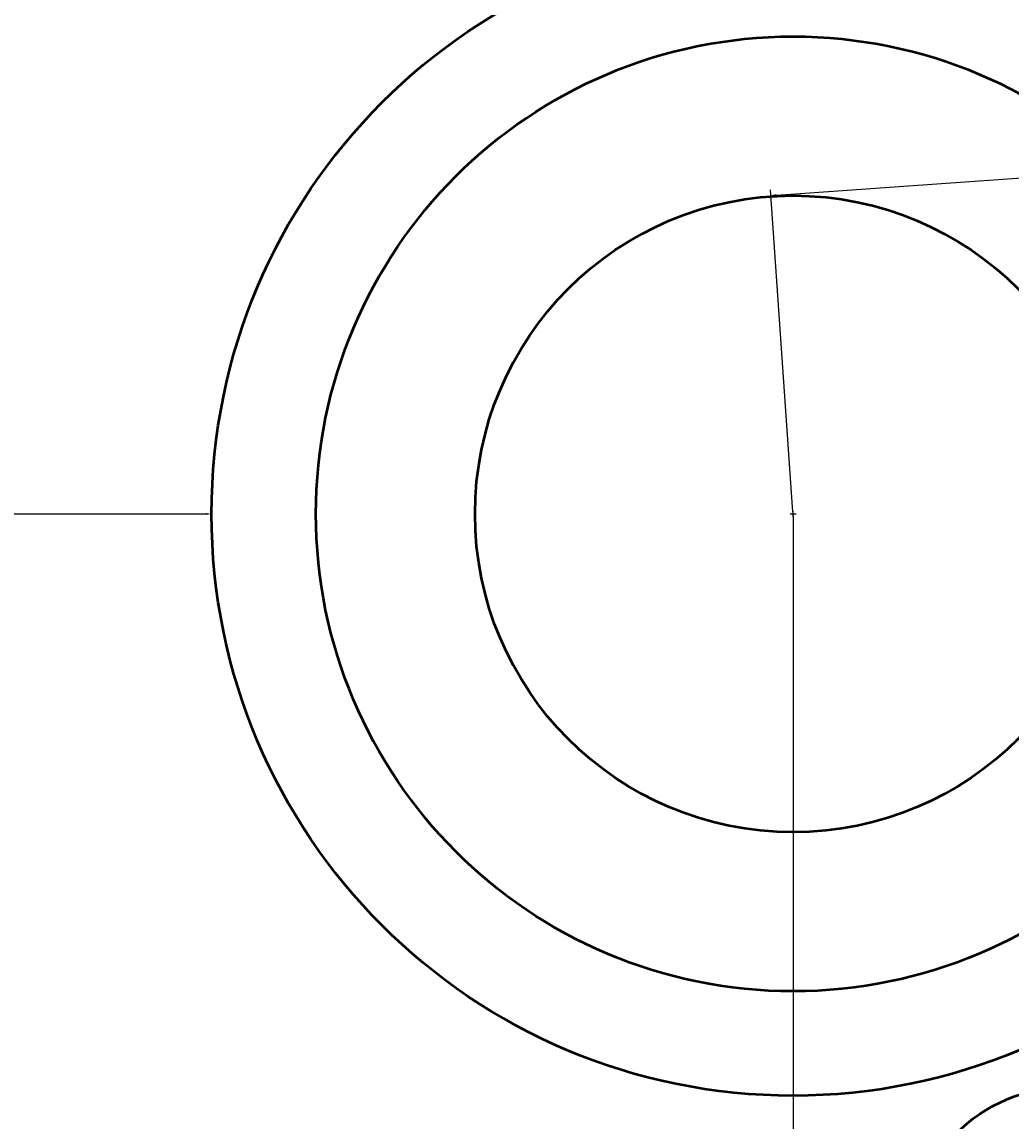
# Model space of a CAD drawing. Units: inches. Extents: x 413 to 622, y 326 to 447.
# Tile 12 of 15: x 568 to 600, y 367 to 402. Entities that reach past the tile are written whole.
import ezdxf

# ---------------------------------------------------------------- set-up
doc = ezdxf.new("R2010")
doc.units = ezdxf.units.IN
doc.header["$MEASUREMENT"] = 0
doc.layers.add('M-DIMS', color=2, linetype='Continuous', lineweight=18)
doc.layers.add('M-OUTL', color=7, linetype='Continuous', lineweight=50)
doc.styles.get("Standard").update_dxf_attribs({"font": 'arial.ttf'})
doc.dimstyles.get("Standard").update_dxf_attribs({"dimtxt": 0.18, "dimasz": 0.18, "dimexe": 0.18, "dimexo": 0.0625, "dimgap": 0.09, "dimtad": 0, "dimtih": 1, "dimtoh": 1, "dimdec": 4, "dimzin": 0, "dimdsep": 46, "dimtxsty": 'Standard', "dimcen": 0.09, "dimadec": 0, "dimazin": 0, "dimtfac": 1, "dimtdec": 4, "dimtofl": 0, "dimtmove": 0, "dimatfit": 3, "dimfxl": 1, "dimtolj": 1, "dimtzin": 0, "dimarcsym": 0})

# ---------------------------------------------------------------- blocks, each defined once
blk = doc.blocks.new('CHAIN-ROLLER-PIN')
for radius in [5, 2.5]:
    blk.add_circle((5, 5), radius)
blk = doc.blocks.new('SPROCKET-HUB-BORE')
for radius in [15, 10]:
    blk.add_circle((15, 15), radius)
blk = doc.blocks.new('*D11')
at = {"layer": 'Defpoints', "color": 0, "transparency": 16777216}
for p in [(621.66, 446.422), (621.66, 388.074), (423.314, 378.888)]:
    blk.add_point(p, dxfattribs=at)
at = {"layer": 'M-DIMS', "color": 0, "lineweight": -2, "transparency": 16777216}
for p, q in [((423.314, 378.95), (423.314, 446.602)), ((621.66, 388.137), (621.66, 446.602)), ((423.494, 446.422), (522.031, 446.422)), ((621.48, 446.422), (522.943, 446.422))]:
    blk.add_line(p, q, dxfattribs=at)
at = {"layer": 'M-DIMS', "color": 0, "transparency": 16777216}
for points in [[(423.494, 446.452), (423.494, 446.392), (423.314, 446.422)], [(621.48, 446.452), (621.48, 446.392), (621.66, 446.422)]]:
    blk.add_solid(points, dxfattribs=at)
at = {"layer": 'M-DIMS', "color": 0, "transparency": 16777216, "insert": (522.487, 446.422), "char_height": 0.18, "attachment_point": 5}
blk.add_mtext('\\A1;198.35', dxfattribs=at)
blk = doc.blocks.new('*D12')
at = {"layer": 'Defpoints', "color": 0, "transparency": 16777216}
for p in [(472.684, 386.392), (592.684, 386.392), (592.684, 326.361)]:
    blk.add_point(p, dxfattribs=at)
at = {"layer": 'M-DIMS', "color": 0, "lineweight": -2, "transparency": 16777216}
for p, q in [((472.684, 386.329), (472.684, 326.181)), ((592.684, 386.329), (592.684, 326.181)), ((472.864, 326.361), (532.404, 326.361)), ((592.504, 326.361), (532.964, 326.361))]:
    blk.add_line(p, q, dxfattribs=at)
at = {"layer": 'M-DIMS', "color": 0, "transparency": 16777216}
for points in [[(472.864, 326.391), (472.864, 326.331), (472.684, 326.361)], [(592.504, 326.391), (592.504, 326.331), (592.684, 326.361)]]:
    blk.add_solid(points, dxfattribs=at)
at = {"layer": 'M-DIMS', "color": 0, "transparency": 16777216, "insert": (532.684, 326.361), "char_height": 0.18, "attachment_point": 5}
blk.add_mtext('\\A1;120', dxfattribs=at)
blk = doc.blocks.new('*D15')
at = {"layer": 'Defpoints', "color": 0, "transparency": 16777216}
for p in [(615.958, 398.08), (616.66, 388.074), (592.684, 386.392)]:
    blk.add_point(p, dxfattribs=at)
at = {"layer": 'M-DIMS', "color": 0, "lineweight": -2, "transparency": 16777216}
for p, q in [((616.656, 388.136), (615.945, 398.26)), ((615.778, 398.067), (604.435, 397.271)), ((592.161, 396.41), (603.504, 397.206)), ((592.679, 386.454), (591.969, 396.577))]:
    blk.add_line(p, q, dxfattribs=at)
at = {"layer": 'M-DIMS', "color": 0, "transparency": 16777216}
for points in [[(615.776, 398.097), (615.78, 398.037), (615.958, 398.08)], [(592.159, 396.44), (592.163, 396.38), (591.981, 396.397)]]:
    blk.add_solid(points, dxfattribs=at)
at = {"layer": 'M-DIMS', "color": 0, "transparency": 16777216, "insert": (603.97, 397.239), "char_height": 0.18, "attachment_point": 5}
blk.add_mtext('\\A1;24.035', dxfattribs=at)
blk = doc.blocks.new('*D25')
at = {"layer": 'Defpoints', "color": 0, "transparency": 16777216}
for p in [(574.404, 386.392), (610.964, 386.391)]:
    blk.add_point(p, dxfattribs=at)
at = {"layer": 'M-DIMS', "color": 0, "lineweight": -2, "transparency": 16777216}
for p, q in [((592.684, 386.302), (592.684, 386.482)), ((563.436, 386.392), (574.224, 386.392)), ((592.594, 386.392), (592.774, 386.392))]:
    blk.add_line(p, q, dxfattribs=at)
at = {"layer": 'M-DIMS', "color": 0, "transparency": 16777216}
blk.add_solid([(574.224, 386.422), (574.224, 386.362), (574.404, 386.392)], dxfattribs=at)
at = {"layer": 'M-DIMS', "color": 0, "transparency": 16777216, "insert": (562.944, 386.392), "char_height": 0.18, "attachment_point": 5}
blk.add_mtext('\\A1;∅36.56', dxfattribs=at)

msp = doc.modelspace()

# ---------------------------------------------------------------- linework, layer by layer
at = {"layer": 'M-OUTL'}
msp.add_circle((592.6836, 386.3915), 18.28, dxfattribs=at)

# ---------------------------------------------------------------- block references
for name, p in [('SPROCKET-HUB-BORE', (577.684, 371.392)), ('CHAIN-ROLLER-PIN', (596.3385, 358.386))]:
    msp.add_blockref(name, p, dxfattribs=at)

# ---------------------------------------------------------------- dimensions: what is measured, and where the dimension line sits
at = {"layer": 'M-DIMS'}
for base, p1, p2, override, picture, middle in [((621.66, 446.422), (423.3136, 378.8878), (621.66, 388.0741), {"dimdec": 2, "dimlfac": 1, "dimrnd": 0, "dimzin": 0, "dimdsep": 46, "dimlunit": 2}, '*D11', (522.4868, 446.422)), ((592.6836, 326.361), (472.6836, 386.3915), (592.6836, 386.3915), {"dimdec": 0, "dimlfac": 1, "dimrnd": 0, "dimzin": 0, "dimdsep": 46, "dimlunit": 2}, '*D12', (532.6836, 326.361))]:
    dim = msp.add_linear_dim(base=base, p1=p1, p2=p2, dimstyle='Standard', override=override, dxfattribs=at)
    dim.commit()
    dim.dimension.update_dxf_attribs({"geometry": picture, "text_midpoint": middle})
dim = msp.add_linear_dim(base=(615.9578, 398.08), p1=(592.6836, 386.3915), p2=(616.66, 388.0741), angle=4.01433, dimstyle='Standard', override={"dimdec": 3, "dimlfac": 1, "dimrnd": 0, "dimzin": 0, "dimdsep": 46, "dimlunit": 2}, dxfattribs=at)
dim.commit()
dim.dimension.update_dxf_attribs({"geometry": '*D15', "text_midpoint": (603.9696, 397.2387)})
dim = msp.add_diameter_dim_2p(p1=(610.9636, 386.391), p2=(574.4036, 386.392), dimstyle='Standard', override={"dimdec": 2, "dimlfac": 1, "dimrnd": 0, "dimzin": 0, "dimdsep": 46, "dimlunit": 2}, dxfattribs=at)
dim.commit()
dim.dimension.update_dxf_attribs({"geometry": '*D25', "text_midpoint": (563.4356, 386.3923), "dimtype": 163})

doc.saveas('drawing.dxf')
